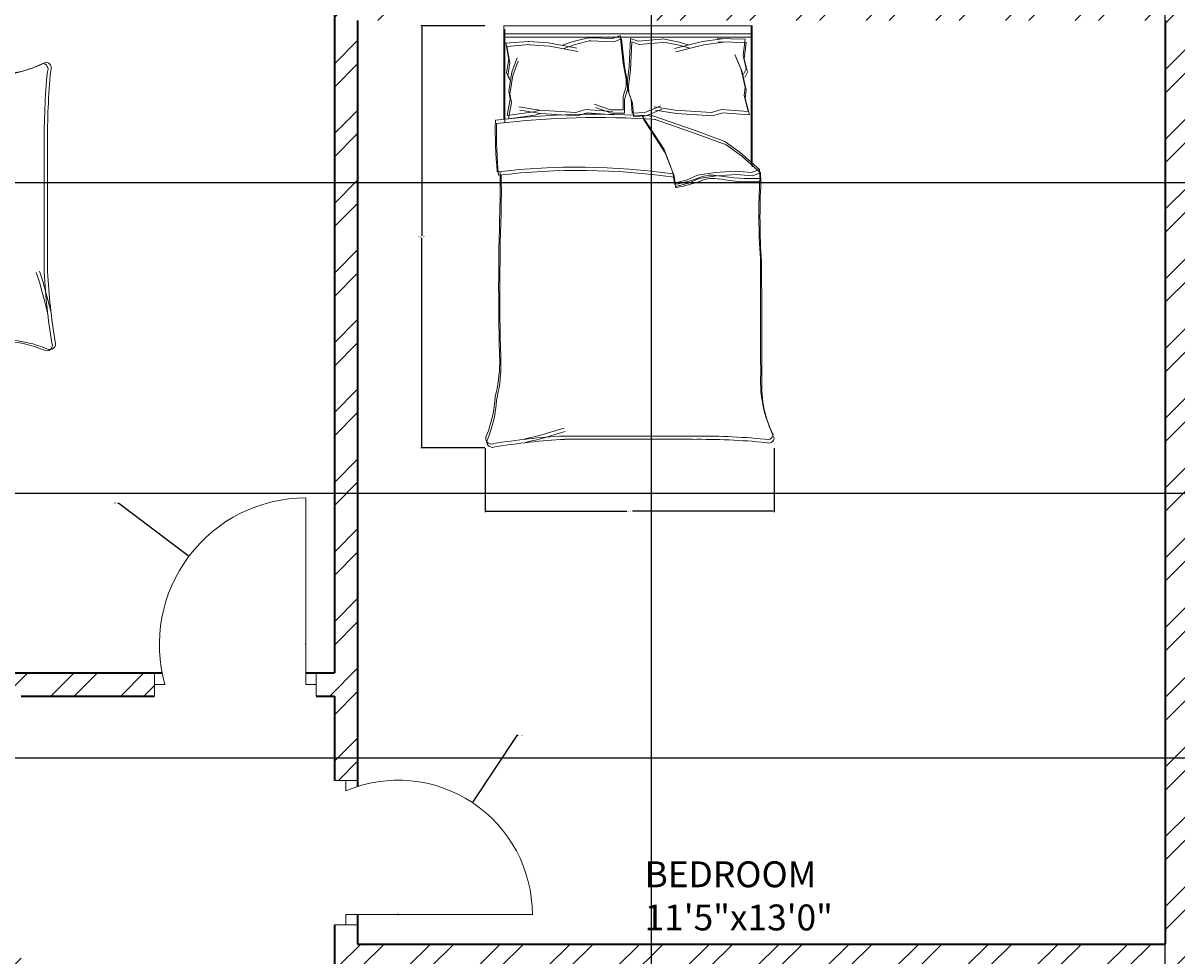
# Model space of a CAD drawing. Units: inches. Extents: x 2008 to 2657, y 1077 to 2165.
# Tile 12 of 16: x 2186 to 2409, y 1845 to 2025. Entities that reach past the tile are written whole.
import ezdxf

# ---------------------------------------------------------------- set-up
doc = ezdxf.new("R2010")
doc.units = ezdxf.units.IN
for name, color, linetype, lineweight in [('A-ANNO-DIMS', 2, 'Continuous', 18), ('A-AREA-IDEN', 4, 'Continuous', 18), ('A-DOOR', 11, 'Continuous', 18), ('A-FURN', 8, 'Continuous', 13), ('A-WALL', 7, 'Continuous', 35)]:
    doc.layers.add(name, color=color, linetype=linetype, lineweight=lineweight)
doc.layers.add('A-WALL-PATT', color=30, linetype='Continuous', lineweight=13, true_color=0xf8991e)
doc.styles.get("Standard").update_dxf_attribs({"font": 'arial.ttf'})
doc.dimstyles.get("Standard").update_dxf_attribs({"dimtxt": 0.18, "dimasz": 0.18, "dimexe": 0.18, "dimexo": 0.0625, "dimgap": 0.09, "dimtad": 0, "dimtih": 1, "dimtoh": 1, "dimdec": 4, "dimzin": 0, "dimdsep": 46, "dimtxsty": 'Standard', "dimcen": 0.09, "dimadec": 0, "dimazin": 0, "dimtfac": 1, "dimtdec": 4, "dimtofl": 0, "dimtmove": 0, "dimatfit": 3, "dimfxl": 1, "dimtolj": 1, "dimtzin": 0, "dimarcsym": 0})

# ---------------------------------------------------------------- blocks, each defined once
blk = doc.blocks.new('BED-DOUBLE')
for p, q in [((0, 51.49), (0.64, 51.49)), ((0, 3.48), (0, 51.49)), ((0, 51.27), (26.61, 51.27)), ((0, 51.27), (26.61, 51.27)), ((0.64, 51.49), (27.25, 51.49)), ((0.64, 51.49), (27.25, 51.49)), ((1.53, 3.48), (1.53, 51.27)), ((1.53, 3.48), (1.53, 51.27)), ((2.17, 3.7), (2.17, 51.49)), ((2.17, 3.7), (2.17, 51.49)), ((27.75, 52.87), (24.5, 49.16)), ((27.75, 52.87), (24.5, 49.16)), ((28.39, 53.1), (25.14, 49.39)), ((28.39, 53.1), (25.14, 49.39)), ((29.49, 52.95), (27.75, 52.87, 3.87)), ((29.49, 52.95), (27.75, 52.87, 3.87)), ((28.37, 51.33), (27.75, 52.87)), ((28.37, 51.33), (27.75, 52.87)), ((28.06, 48.23), (28.37, 51.33)), ((28.06, 48.23), (28.37, 51.33)), ((30.13, 53.18), (28.39, 53.1, 3.87)), ((30.13, 53.18), (28.39, 53.1, 3.87)), ((29, 51.56), (28.39, 53.1)), ((29, 51.56), (28.39, 53.1)), ((28.7, 48.46), (29, 51.56)), ((28.7, 48.46), (29, 51.56)), ((2.56, 50.11), (2.46, 44.71)), ((2.56, 50.11), (2.46, 44.71)), ((2.56, 50.11), (5.77, 49.73)), ((2.56, 50.11), (5.77, 49.73)), ((3.2, 50.34), (3.1, 44.94)), ((3.2, 50.34), (3.1, 44.94)), ((3.2, 50.34), (6.41, 49.96)), ((3.2, 50.34), (6.41, 49.96)), ((8.26, 49.31), (5.58, 48.13)), ((8.26, 49.31), (5.58, 48.13)), ((5.77, 49.73), (8.34, 50.33)), ((5.77, 49.73), (8.34, 50.33)), ((8.9, 49.54), (6.22, 48.36)), ((8.9, 49.54), (6.22, 48.36)), ((6.41, 49.96), (8.98, 50.56)), ((6.41, 49.96), (8.98, 50.56)), ((11.83, 50.11), (8.26, 49.31)), ((11.83, 50.11), (8.26, 49.31)), ((8.34, 50.33), (9.38, 49.82)), ((8.34, 50.33), (9.38, 49.81)), ((12.47, 50.34), (8.9, 49.54)), ((12.47, 50.34), (8.9, 49.54)), ((8.98, 50.56), (10.02, 50.04)), ((8.98, 50.56), (10.02, 50.04)), ((13.43, 49.92), (11.83, 50.11)), ((13.43, 49.92), (11.83, 50.11)), ((14.07, 50.15), (12.47, 50.34)), ((14.07, 50.15), (12.47, 50.34)), ((16.57, 50.7), (13.43, 49.92)), ((16.57, 50.7), (13.43, 49.92)), ((17.21, 50.93), (14.07, 50.15)), ((17.21, 50.93), (14.07, 50.15)), ((16.17, 45.57), (16.57, 50.7)), ((16.17, 45.57), (16.57, 50.7)), ((16.81, 45.8), (17.21, 50.93)), ((16.81, 45.8), (17.21, 50.93)), ((24.5, 49.16), (22.33, 46.22)), ((24.5, 49.16), (22.33, 46.22)), ((25.14, 49.39), (22.97, 46.45)), ((25.14, 49.39), (22.97, 46.45)), ((28.37, 44.36), (28.06, 48.23)), ((28.37, 44.36), (28.06, 48.23)), ((29, 44.59), (28.7, 48.46)), ((29, 44.59), (28.7, 48.46)), ((2.46, 44.71), (2.54, 45.71)), ((2.46, 44.71), (2.54, 45.71)), ((2.54, 45.71), (3.07, 41.91)), ((2.54, 45.71), (3.07, 41.91)), ((3.1, 44.94), (3.18, 45.94)), ((3.1, 44.94), (3.18, 45.94)), ((3.18, 45.94), (3.71, 42.14)), ((3.18, 45.94), (3.71, 42.14)), ((16.73, 43.61), (16.17, 45.57)), ((16.73, 43.61), (16.17, 45.57)), ((17.37, 43.84), (16.81, 45.8)), ((17.37, 43.83), (16.81, 45.8)), ((22.33, 46.22), (20.32, 40.64)), ((22.33, 46.22), (20.32, 40.64)), ((22.97, 46.45), (20.96, 40.87)), ((22.97, 46.45), (20.96, 40.87)), ((29.47, 41.18), (29, 44.59)), ((29.47, 41.18), (29, 44.59)), ((16.3, 36.6), (16.73, 43.61)), ((16.3, 36.6), (16.73, 43.61)), ((16.93, 36.83), (17.37, 43.84)), ((16.93, 36.82), (17.37, 43.83)), ((28.83, 40.95), (28.37, 44.36)), ((28.83, 40.95), (28.37, 44.36)), ((3.07, 41.91), (4.42, 36.5)), ((3.07, 41.91), (4.42, 36.5)), ((3.71, 42.14), (5.06, 36.72)), ((3.71, 42.14), (5.06, 36.72)), ((20.32, 40.64), (17.38, 32.31)), ((20.32, 40.64), (17.38, 32.31)), ((20.96, 40.87), (18.02, 32.54)), ((20.96, 40.87), (18.02, 32.53)), ((29.76, 38.94), (28.83, 40.95)), ((29.76, 38.94), (28.83, 40.95)), ((30.4, 39.17), (29.47, 41.18)), ((30.4, 39.17), (29.47, 41.18)), ((3.67, 39.2), (3.08, 37.14)), ((3.67, 39.2), (3.08, 37.14)), ((4.31, 39.43), (3.72, 37.36)), ((4.31, 39.43), (3.72, 37.36)), ((30.38, 36.46), (29.76, 38.94)), ((30.38, 36.46), (29.76, 38.94)), ((31.02, 36.69), (30.4, 39.17)), ((31.02, 36.69), (30.4, 39.17)), ((79.25, 15.06), (79.25, 39.68)), ((79.25, 15.06), (79.25, 39.68)), ((79.88, 15.29), (79.88, 39.91)), ((79.88, 15.29), (79.88, 39.91)), ((3.08, 37.14), (2.54, 34.21)), ((3.08, 37.14), (2.54, 34.2)), ((3.72, 37.36), (3.18, 34.43)), ((3.72, 37.36), (3.18, 34.43)), ((15.63, 32.56), (16.3, 36.6)), ((15.63, 32.56), (16.3, 36.6)), ((16.27, 32.79), (16.93, 36.83)), ((16.27, 32.79), (16.93, 36.82)), ((23.88, 34.45), (28.37, 36.15)), ((23.88, 34.45), (28.37, 36.15)), ((24.52, 34.68), (29, 36.38)), ((24.52, 34.68), (29, 36.38)), ((28.37, 36.15), (30.38, 36.46)), ((28.37, 36.15), (30.38, 36.46)), ((29, 36.38), (31.02, 36.69)), ((29, 36.38), (31.02, 36.69)), ((2.54, 34.21), (2.56, 33.88)), ((2.54, 34.2), (2.56, 33.88)), ((2.56, 33.88), (2.98, 29.46)), ((2.56, 33.88), (2.98, 29.46)), ((3.18, 34.43), (3.2, 34.11)), ((3.18, 34.43), (3.2, 34.11)), ((3.2, 34.11), (3.62, 29.68)), ((3.2, 34.11), (3.62, 29.68)), ((16.74, 30.75), (15.45, 33.82)), ((16.74, 30.75), (15.45, 33.82)), ((17.38, 30.98), (16.09, 34.05)), ((17.38, 30.98), (16.09, 34.05)), ((17.38, 30.26), (23.88, 34.45)), ((17.38, 30.26), (23.88, 34.45)), ((18.02, 30.49), (24.52, 34.68)), ((18.02, 30.49), (24.52, 34.68)), ((2.98, 29.46), (2.49, 27.98)), ((2.98, 29.46), (2.49, 27.98)), ((3.62, 29.68), (3.13, 28.21)), ((3.62, 29.68), (3.13, 28.21)), ((16.89, 28.3), (16.74, 30.75)), ((16.89, 28.3), (16.74, 30.75)), ((17.53, 28.53), (17.38, 30.98)), ((17.53, 28.53), (17.38, 30.98)), ((2.49, 27.98), (7.87, 27.73)), ((2.49, 27.98), (7.87, 27.73)), ((2.51, 26.21), (7.86, 26.79)), ((2.51, 26.21), (7.86, 26.79)), ((3.13, 28.21), (8.51, 27.96)), ((3.13, 28.21), (8.51, 27.96)), ((7.22, 26.56), (10.4, 27.14)), ((7.22, 26.56), (10.4, 27.14)), ((7.86, 26.79), (11.04, 27.37)), ((7.86, 26.79), (11.04, 27.37)), ((7.87, 27.73), (11.08, 27.36)), ((7.87, 27.73), (11.08, 27.36)), ((8.51, 27.96), (11.72, 27.58)), ((8.51, 27.96), (11.72, 27.58)), ((10.4, 27.14), (11.7, 27.14)), ((10.4, 27.14), (11.7, 27.14)), ((11.04, 27.37), (12.34, 27.37)), ((11.04, 27.37), (12.34, 27.37)), ((11.08, 27.36), (12.38, 27.44)), ((11.08, 27.36), (12.38, 27.44)), ((11.7, 27.14), (13.58, 26.56)), ((11.7, 27.14), (13.58, 26.56)), ((11.72, 27.58), (13.02, 27.66)), ((11.72, 27.58), (13.02, 27.66)), ((12.34, 27.37), (14.22, 26.79)), ((12.34, 27.37), (14.22, 26.79)), ((12.38, 27.44), (14.22, 28.13)), ((12.38, 27.44), (14.22, 28.13)), ((13.02, 27.66), (14.86, 28.36)), ((13.02, 27.66), (14.86, 28.36)), ((14.22, 28.13), (16.89, 28.3)), ((14.22, 28.13), (16.89, 28.3)), ((14.22, 26.79), (16.9, 26.79)), ((14.22, 26.79), (16.9, 26.79)), ((14.86, 28.36), (17.53, 28.53)), ((14.86, 28.36), (17.53, 28.53)), ((16.9, 26.79), (16.9, 24.33)), ((16.9, 26.79), (16.9, 24.33)), ((1.87, 25.98), (7.22, 26.56)), ((1.87, 25.98), (7.22, 26.56)), ((2.45, 24.54), (1.87, 25.98)), ((2.45, 24.54), (1.87, 25.98)), ((2.3, 20.09), (2.45, 24.54)), ((2.3, 20.09), (2.45, 24.54)), ((3.09, 24.77), (2.51, 26.21)), ((3.09, 24.77), (2.51, 26.21)), ((2.94, 20.32), (3.09, 24.77)), ((2.94, 20.32), (3.09, 24.77)), ((13.58, 26.56), (16.26, 26.56)), ((13.58, 26.56), (16.26, 26.56)), ((16.17, 19.38), (16.57, 24.52)), ((16.17, 19.38), (16.57, 24.52)), ((16.26, 26.56), (16.26, 24.1)), ((16.26, 26.56), (16.26, 24.1)), ((16.81, 19.61), (17.21, 24.74)), ((16.81, 19.61), (17.21, 24.74)), ((16.26, 24.1), (15.17, 20.96)), ((16.26, 24.1), (15.17, 20.96)), ((16.9, 24.33), (15.81, 21.19)), ((16.9, 24.33), (15.81, 21.19)), ((2.3, 19.77), (2.3, 20.09)), ((2.3, 19.77), (2.3, 20.09)), ((2.94, 20), (2.94, 20.32)), ((2.94, 20), (2.94, 20.32)), ((3.03, 16.88), (2.3, 19.77)), ((3.03, 16.88), (2.3, 19.77)), ((3.67, 17.11), (2.94, 20)), ((3.67, 17.11), (2.94, 20)), ((3.96, 12.34), (4.97, 17.83)), ((3.96, 12.34), (4.97, 17.83)), ((16.73, 17.42), (16.17, 19.38)), ((16.73, 17.42), (16.17, 19.38)), ((17.37, 17.65), (16.81, 19.61)), ((17.37, 17.65), (16.81, 19.61)), ((3.75, 14.86), (3.03, 16.88)), ((3.75, 14.86), (3.03, 16.88)), ((3.32, 12.11), (4.33, 17.6)), ((3.32, 12.11), (4.33, 17.6)), ((4.39, 15.08), (3.67, 17.11)), ((4.39, 15.08), (3.67, 17.11)), ((16.3, 10.41), (16.73, 17.42)), ((16.3, 10.41), (16.73, 17.42)), ((16.93, 10.64), (17.37, 17.65)), ((16.93, 10.64), (17.37, 17.65)), ((3.03, 8.29), (3.32, 12.11)), ((3.03, 8.29), (3.32, 12.11)), ((3.67, 8.51), (3.96, 12.34)), ((3.67, 8.51), (3.96, 12.34)), ((15.63, 6.38), (16.3, 10.41)), ((15.63, 6.38), (16.3, 10.41)), ((16.27, 6.61), (16.93, 10.64)), ((16.27, 6.61), (16.93, 10.64)), ((16.3, 10.41), (16.62, 9.28)), ((16.3, 10.41), (16.62, 9.28)), ((16.62, 9.28), (17.34, 4.18)), ((16.62, 9.28), (17.34, 4.18)), ((16.93, 10.64), (17.26, 9.51)), ((16.93, 10.64), (17.26, 9.51)), ((17.26, 9.51), (17.98, 4.41)), ((17.26, 9.51), (17.98, 4.41)), ((3.01, 8.18), (3.03, 8.29)), ((3.01, 8.18), (3.03, 8.29)), ((3.34, 3.9), (3.01, 8.18)), ((3.34, 3.9), (3.01, 8.18)), ((3.65, 8.41), (3.67, 8.51)), ((3.65, 8.41), (3.67, 8.51)), ((3.98, 4.13), (3.65, 8.41)), ((3.98, 4.13), (3.65, 8.41)), ((3.32, 3.9), (6.5, 4.47)), ((3.32, 3.89), (6.5, 4.47)), ((3.96, 4.12), (7.14, 4.7)), ((3.96, 4.12), (7.14, 4.7)), ((8.96, 5.05), (6.21, 6.06)), ((8.96, 5.05), (6.21, 6.06)), ((6.5, 4.47), (9.1, 4.04)), ((6.5, 4.47), (9.1, 4.04)), ((9.59, 5.28), (6.85, 6.29)), ((9.59, 5.28), (6.85, 6.29)), ((7.14, 4.7), (9.74, 4.27)), ((7.14, 4.7), (9.74, 4.27)), ((12.57, 4.47), (8.96, 5.05)), ((12.57, 4.47), (8.96, 5.05)), ((9.1, 4.04), (10.11, 4.62)), ((9.1, 4.04), (10.11, 4.62)), ((13.21, 4.7), (9.59, 5.28)), ((13.21, 4.7), (9.59, 5.28)), ((9.74, 4.27), (10.75, 4.85)), ((9.74, 4.27), (10.75, 4.85)), ((14.16, 4.76), (12.57, 4.47)), ((14.16, 4.76), (12.57, 4.47)), ((14.8, 4.99), (13.21, 4.7)), ((14.8, 4.99), (13.21, 4.7)), ((17.34, 4.18), (14.16, 4.76)), ((17.34, 4.18), (14.16, 4.76)), ((17.98, 4.41), (14.8, 4.99)), ((17.98, 4.41), (14.8, 4.99)), ((18.11, 3.48), (0, 3.48)), ((18.11, 3.48), (0, 3.48)), ((18.75, 3.7), (0.64, 3.7)), ((18.75, 3.7), (0.64, 3.7))]:
    blk.add_line(p, q)
for centre, radius, start, end in [((69.31, 76.39), 23.07, 267.4714, 296.4681), ((69.31, 76.39), 23.07, 267.4714, 296.4681), ((79.51, 54.64), 1.1, 332.6588, 86.02), ((79.51, 54.64), 1.1, 332.6588, 86.02), ((68.67, 76.16), 23.07, 267.4714, 296.4681), ((68.67, 76.16), 23.07, 267.4714, 296.4681), ((78.87, 54.41), 1.1, 332.6588, 86.02), ((78.87, 54.41), 1.1, 332.6588, 86.02), ((212.28, 41.15), 133.04, 174.4998, 180.6351), ((212.28, 41.15), 133.04, 174.4998, 180.6351), ((212.92, 41.38), 133.04, 174.4998, 180.6351), ((212.92, 41.38), 133.04, 174.4998, 180.6351), ((-6.66, 51.33), 36.18, 349.8763, 2.5657), ((-6.66, 51.33), 36.18, 349.8763, 2.5657), ((36.32, 182.27), 129.5, 266.9791, 273.8365), ((36.32, 182.27), 129.5, 266.9791, 273.8365), ((-6.02, 51.56), 36.18, 349.8763, 2.5657), ((-6.02, 51.56), 36.18, 349.8763, 2.5657), ((36.95, 182.49), 129.5, 266.9791, 273.8365), ((36.95, 182.49), 129.5, 266.9791, 273.8365), ((67.82, -4508.74), 4561.86, 90.00217, 90.28689), ((67.82, -4508.74), 4561.86, 90.00217, 90.28689), ((68.46, -4508.51), 4561.86, 90.00217, 90.28689), ((68.46, -4508.51), 4561.86, 90.00217, 90.28689), ((35.07, 43.74), 6.22, 168.6608, 203.7384), ((35.07, 43.74), 6.22, 168.6608, 203.7384), ((35.71, 43.97), 6.22, 168.6608, 203.7384), ((35.71, 43.97), 6.22, 168.6608, 203.7384), ((1.48, 31.15), 29.65, 10.6617, 19.8806), ((1.48, 31.15), 29.65, 10.6617, 19.8806), ((2.12, 31.38), 29.65, 10.6617, 19.8806), ((2.12, 31.38), 29.65, 10.6617, 19.8806), ((156.32, 17.76), 129.02, 171.7845, 186.9006), ((156.32, 17.76), 129.02, 171.7845, 186.9006), ((156.96, 17.98), 129.02, 171.7845, 186.9006), ((156.96, 17.98), 129.02, 171.7845, 186.9006), ((30.44, 36.64), 0.185, 250.2464, 1.1377), ((30.44, 36.64), 0.185, 250.2464, 1.1377), ((31.08, 36.87), 0.185, 250.2464, 1.1377), ((31.08, 36.86), 0.185, 250.2464, 1.1377), ((182.05, 21.36), 164.97, 176.0865, 186.7821), ((182.05, 21.36), 164.97, 176.0865, 186.7821), ((182.69, 21.59), 164.97, 176.0865, 186.7821), ((182.69, 21.59), 164.97, 176.0865, 186.7821), ((-23.71, -17.22), 106.46, 13.3832, 17.7053), ((-23.71, -17.22), 106.46, 13.3832, 17.7053), ((-23.07, -16.99), 106.46, 13.3832, 17.7053), ((-23.07, -16.99), 106.46, 13.3832, 17.7053), ((200.84, 21.43), 121.76, 182.9958, 189.4091), ((200.84, 21.43), 121.76, 182.9958, 189.4091), ((201.48, 21.66), 121.76, 182.9958, 189.4091), ((201.48, 21.66), 121.76, 182.9958, 189.4091), ((20.1, 85.16), 83.31, 268.7218, 275.604), ((20.1, 85.16), 83.31, 268.7218, 275.604), ((20.74, 85.39), 83.31, 268.7218, 275.604), ((20.74, 85.39), 83.31, 268.7218, 275.604), ((31.17, -167.31), 170.11, 88.4762, 91.0082), ((31.17, -167.31), 170.11, 88.4762, 91.0082), ((31.81, -167.08), 170.11, 88.4762, 91.0082), ((31.81, -167.08), 170.11, 88.4762, 91.0082), ((50.61, 484.82), 482.31, 268.2277, 271.7185), ((50.61, 484.82), 482.31, 268.2277, 271.7185), ((51.25, 485.05), 482.31, 268.2277, 271.7185), ((51.25, 485.05), 482.31, 268.2277, 271.7185), ((64.52, -26.9), 29.63, 76.0648, 88.9113), ((64.52, -26.9), 29.63, 76.0648, 88.9113), ((65.15, -26.67), 29.63, 76.0648, 88.9113), ((65.15, -26.67), 29.63, 76.0648, 88.9113), ((70.28, -21.66), 23.56, 67.9751, 86.652), ((70.28, -21.66), 23.56, 67.9751, 86.652), ((70.92, -21.43), 23.56, 67.9751, 86.652), ((70.92, -21.43), 23.56, 67.9751, 86.652), ((79.72, 1.09), 1.09, 236.1736, 23.4781), ((79.72, 1.09), 1.09, 236.1736, 23.4781), ((80.36, 1.32), 1.09, 236.1736, 23.4781), ((80.36, 1.32), 1.09, 236.1736, 23.4781)]:
    blk.add_arc(centre, radius, start, end)
blk = doc.blocks.new('*D11')
at = {"layer": 'A-ANNO-DIMS', "color": 0, "lineweight": -2, "transparency": 16777216}
for p, q in [((2275.34, 2024.63), (2262.99, 2024.63)), ((2263.17, 2024.45), (2263.17, 1984.04)), ((2263.17, 1943.27), (2263.17, 1983.68)), ((2275.34, 1943.09), (2262.99, 1943.09))]:
    blk.add_line(p, q, dxfattribs=at)
at = {"layer": 'A-ANNO-DIMS', "color": 0, "transparency": 16777216}
for points in [[(2263.14, 2024.45), (2263.2, 2024.45), (2263.17, 2024.63)], [(2263.14, 1943.27), (2263.2, 1943.27), (2263.17, 1943.09)]]:
    blk.add_solid(points, dxfattribs=at)
at = {"layer": 'Defpoints', "color": 0, "transparency": 16777216}
for p in [(2275.4, 2024.63), (2263.17, 1943.09), (2275.4, 1943.09)]:
    blk.add_point(p, dxfattribs=at)
at = {"layer": 'A-ANNO-DIMS', "color": 0, "transparency": 16777216, "insert": (2263.17, 1983.86), "char_height": 0.18, "attachment_point": 5}
blk.add_mtext('\\A1;BED 82 TYP.', dxfattribs=at)
blk = doc.blocks.new('*D12')
at = {"layer": 'A-ANNO-DIMS', "color": 0, "lineweight": -2, "transparency": 16777216}
for p, q in [((2275.4, 1943.02), (2275.4, 1930.67)), ((2331.23, 1943.02), (2331.23, 1930.67)), ((2275.58, 1930.85), (2302.79, 1930.85)), ((2331.05, 1930.85), (2303.84, 1930.85))]:
    blk.add_line(p, q, dxfattribs=at)
at = {"layer": 'A-ANNO-DIMS', "color": 0, "transparency": 16777216}
for points in [[(2275.58, 1930.88), (2275.58, 1930.82), (2275.4, 1930.85)], [(2331.05, 1930.88), (2331.05, 1930.82), (2331.23, 1930.85)]]:
    blk.add_solid(points, dxfattribs=at)
at = {"layer": 'Defpoints', "color": 0, "transparency": 16777216}
for p in [(2275.4, 1943.09), (2331.23, 1943.09), (2331.23, 1930.85)]:
    blk.add_point(p, dxfattribs=at)
at = {"layer": 'A-ANNO-DIMS', "color": 0, "transparency": 16777216, "insert": (2303.32, 1930.85), "char_height": 0.18, "attachment_point": 5}
blk.add_mtext('\\A1;56 TYP.', dxfattribs=at)
blk = doc.blocks.new('*D51')
at = {"layer": 'A-ANNO-DIMS', "color": 0, "lineweight": -2, "transparency": 16777216}
for p, q in [((2307.5, 1617.74), (2307.5, 2142.9)), ((2307.68, 2142.72), (2356.74, 2142.72)), ((2406.58, 2142.72), (2357.53, 2142.72)), ((2406.76, 1617.74), (2406.76, 2142.9))]:
    blk.add_line(p, q, dxfattribs=at)
at = {"layer": 'A-ANNO-DIMS', "color": 0, "transparency": 16777216}
for points in [[(2307.68, 2142.75), (2307.68, 2142.69), (2307.5, 2142.72)], [(2406.58, 2142.75), (2406.58, 2142.69), (2406.76, 2142.72)]]:
    blk.add_solid(points, dxfattribs=at)
at = {"layer": 'Defpoints', "color": 0, "transparency": 16777216}
for p in [(2406.76, 2142.72), (2307.5, 1617.67), (2406.76, 1617.67)]:
    blk.add_point(p, dxfattribs=at)
at = {"layer": 'A-ANNO-DIMS', "color": 0, "transparency": 16777216, "insert": (2357.13, 2142.72), "char_height": 0.18, "attachment_point": 5}
blk.add_mtext('\\A1;99.26', dxfattribs=at)
blk = doc.blocks.new('*D66')
at = {"layer": 'A-ANNO-DIMS', "color": 0, "lineweight": -2, "transparency": 16777216}
for p, q in [((2572.2, 2055.67), (2028.03, 2055.67)), ((2028.21, 2055.49), (2028.21, 2025.16)), ((2028.21, 1994.47), (2028.21, 2024.8)), ((2572.2, 1994.29), (2028.03, 1994.29))]:
    blk.add_line(p, q, dxfattribs=at)
at = {"layer": 'A-ANNO-DIMS', "color": 0, "transparency": 16777216}
for points in [[(2028.18, 2055.49), (2028.24, 2055.49), (2028.21, 2055.67)], [(2028.18, 1994.47), (2028.24, 1994.47), (2028.21, 1994.29)]]:
    blk.add_solid(points, dxfattribs=at)
at = {"layer": 'Defpoints', "color": 0, "transparency": 16777216}
for p in [(2572.26, 2055.67), (2028.21, 1994.29), (2572.26, 1994.29)]:
    blk.add_point(p, dxfattribs=at)
at = {"layer": 'A-ANNO-DIMS', "color": 0, "transparency": 16777216, "insert": (2028.21, 2024.98), "char_height": 0.18, "attachment_point": 5}
blk.add_mtext('\\A1;61.39', dxfattribs=at)
blk = doc.blocks.new('*D67')
at = {"layer": 'A-ANNO-DIMS', "color": 0, "lineweight": -2, "transparency": 16777216}
for p, q in [((2572.2, 1934.29), (2028.03, 1934.29)), ((2028.21, 1934.11), (2028.21, 1908.91)), ((2028.21, 1883.35), (2028.21, 1908.55)), ((2572.2, 1883.17), (2028.03, 1883.17))]:
    blk.add_line(p, q, dxfattribs=at)
at = {"layer": 'A-ANNO-DIMS', "color": 0, "transparency": 16777216}
for points in [[(2028.18, 1934.11), (2028.24, 1934.11), (2028.21, 1934.29)], [(2028.18, 1883.35), (2028.24, 1883.35), (2028.21, 1883.17)]]:
    blk.add_solid(points, dxfattribs=at)
at = {"layer": 'Defpoints', "color": 0, "transparency": 16777216}
for p in [(2028.21, 1934.29), (2572.26, 1934.29), (2572.26, 1883.17)]:
    blk.add_point(p, dxfattribs=at)
at = {"layer": 'A-ANNO-DIMS', "color": 0, "transparency": 16777216, "insert": (2028.21, 1908.73), "char_height": 0.18, "attachment_point": 5}
blk.add_mtext('\\A1;51.11', dxfattribs=at)
blk = doc.blocks.new('*D74')
at = {"layer": 'A-ANNO-DIMS', "color": 0, "lineweight": -2, "transparency": 16777216}
for p, q in [((2204.47, 1932.42), (2204.65, 1932.42)), ((2204.65, 1932.42), (2218.04, 1922.3)), ((2240.66, 1905.15), (2240.84, 1905.15)), ((2240.75, 1905.06), (2240.75, 1905.24))]:
    blk.add_line(p, q, dxfattribs=at)
at = {"layer": 'A-ANNO-DIMS', "color": 0, "transparency": 16777216}
blk.add_solid([(2218.06, 1922.33), (2218.02, 1922.28), (2218.18, 1922.19)], dxfattribs=at)
at = {"layer": 'Defpoints', "color": 0, "transparency": 16777216}
for p in [(2218.18, 1922.19), (2240.75, 1905.15)]:
    blk.add_point(p, dxfattribs=at)
at = {"layer": 'A-ANNO-DIMS', "color": 0, "transparency": 16777216, "insert": (2203.99, 1932.42), "char_height": 0.18, "attachment_point": 5}
blk.add_mtext('\\A1;R28.28', dxfattribs=at)
blk = doc.blocks.new('*D79')
at = {"layer": 'A-ANNO-DIMS', "color": 0, "lineweight": -2, "transparency": 16777216}
for p, q in [((2281.52, 1887.55), (2273.02, 1874.74)), ((2281.7, 1887.55), (2281.52, 1887.55)), ((2258.5, 1852.99), (2258.68, 1852.99)), ((2258.59, 1852.9), (2258.59, 1853.08))]:
    blk.add_line(p, q, dxfattribs=at)
at = {"layer": 'A-ANNO-DIMS', "color": 0, "transparency": 16777216}
blk.add_solid([(2272.99, 1874.76), (2273.04, 1874.72), (2272.92, 1874.59)], dxfattribs=at)
at = {"layer": 'Defpoints', "color": 0, "transparency": 16777216}
for p in [(2272.92, 1874.59), (2258.59, 1852.99)]:
    blk.add_point(p, dxfattribs=at)
at = {"layer": 'A-ANNO-DIMS', "color": 0, "transparency": 16777216, "insert": (2282.25, 1887.55), "char_height": 0.18, "attachment_point": 5}
blk.add_mtext('\\A1;R25.923', dxfattribs=at)

msp = doc.modelspace()

# ---------------------------------------------------------------- hatches: boundary and pattern name
at = {"layer": 'A-WALL-PATT'}
h = msp.add_hatch(dxfattribs=at)
h.set_pattern_fill('ANSI32', color=256)
h.paths.add_polyline_path([(2109.2619, 2094.6743), (2104.7619, 2094.6743), (2104.7619, 2072.1743), (2104.7619, 2021.6151), (2109.2619, 2021.6151), (2109.2619, 2055.6743), (2126.1387, 2055.6743), (2126.1387, 2057.9243), (2126.1387, 2060.1743), (2109.2619, 2060.1743)])
h.paths.add_polyline_path([(2223.2494, 2057.9243), (2223.2494, 2060.1743), (2186.1387, 2060.1743), (2186.1387, 2055.6743), (2223.2494, 2055.6743)])
h.paths.add_polyline_path([(2250.7619, 2072.1743), (2250.7619, 2090.1743), (2250.7619, 2094.6743), (2246.2619, 2094.6743), (2246.2619, 2060.1743), (2242.7242, 2060.1743), (2242.7242, 2055.6743), (2246.2619, 2055.6743), (2246.2619, 1899.6743), (2242.7458, 1899.6743), (2242.7458, 1897.4243), (2242.7458, 1895.1743), (2246.2619, 1895.1743), (2246.2619, 1878.8745), (2248.5119, 1878.8745), (2250.7619, 1878.8745), (2250.7619, 1991.1743), (2250.7619, 2025.6743), (2257.6798, 2025.6743), (2257.6798, 2027.9243), (2257.6798, 2030.1743), (2250.7619, 2030.1743)])
h.paths.add_polyline_path([(2411.2619, 2031.6743), (2409.0119, 2031.6743), (2406.7619, 2031.6743), (2406.7619, 2030.1743), (2322.7619, 2030.1743), (2322.7619, 2053.3443), (2318.2619, 2053.3443), (2318.2619, 2030.1743), (2305.6798, 2030.1743), (2305.6798, 2025.6743), (2318.2619, 2025.6743), (2322.7619, 2025.6743), (2406.7619, 2025.6743), (2406.7619, 1995.6743), (2406.7619, 1847.2677), (2250.7619, 1847.2677), (2250.7619, 1850.9902), (2248.5119, 1850.9902), (2246.2619, 1850.9902), (2246.2619, 1847.1743), (2246.2619, 1842.7677), (2303.0015, 1842.7677), (2303.0015, 1667.2413), (2298.4208, 1667.2413), (2298.4208, 1662.7413), (2303.0015, 1662.7413), (2303.0015, 1649.8758), (2307.5015, 1649.8758), (2307.5015, 1842.7677), (2406.7619, 1842.7677), (2411.2619, 1842.7677), (2411.2619, 1878.6743), (2415.8196, 1878.6743), (2415.8196, 1880.9243), (2415.8196, 1883.1743), (2411.2619, 1883.1743)])
h.paths.add_polyline_path([(2411.2619, 2094.6743), (2406.7619, 2094.6743), (2318.2619, 2094.6743), (2318.2619, 2077.3443), (2322.7619, 2077.3443), (2322.7619, 2090.1743), (2406.7619, 2090.1743), (2406.7619, 2072.1743), (2406.7619, 2067.6743), (2406.7619, 2052.7524), (2411.2619, 2052.7524), (2411.2619, 2055.6743), (2414.9888, 2055.6743), (2414.9888, 2057.9243), (2414.9888, 2060.1743), (2411.2619, 2060.1743), (2411.2619, 2072.1743)])
h.paths.add_polyline_path([(2576.7619, 2072.1743), (2576.7619, 2094.6743), (2572.2619, 2094.6743), (2572.2619, 2060.1743), (2525.8113, 2060.1743), (2525.8113, 2055.6743), (2572.2619, 2055.6743), (2572.2619, 1994.289), (2576.7619, 1994.289)])
h.paths.add_polyline_path([(2465.8113, 2060.1743), (2436.2802, 2060.1743), (2436.2802, 2055.6743), (2465.8113, 2055.6743), (2465.8113, 2057.9243)])
h.paths.add_polyline_path([(2576.7619, 1934.289), (2574.5119, 1934.289), (2572.2619, 1934.289), (2572.2619, 1883.1743), (2447.7027, 1883.1743), (2447.7027, 1878.6743), (2459.7619, 1878.6743), (2459.7619, 1830.4982), (2464.2619, 1830.4982), (2464.2619, 1878.6743), (2572.2619, 1878.6743), (2572.2619, 1868.4883), (2576.7619, 1868.4883)])
h.paths.add_polyline_path([(2576.7619, 1832.4883), (2572.2619, 1832.4883), (2572.2619, 1806.6743), (2464.2619, 1806.6743), (2464.2619, 1809.6629), (2459.7619, 1809.6629), (2459.7619, 1802.1743), (2483.7619, 1802.1743), (2483.7619, 1778.1743), (2488.2619, 1778.1743), (2488.2619, 1802.1743), (2572.2619, 1802.1743), (2572.2619, 1793.6101), (2576.7619, 1793.6101)])
h.paths.add_polyline_path([(2576.7619, 1769.6101), (2572.2619, 1769.6101), (2572.2619, 1754.1743), (2488.2619, 1754.1743), (2488.2619, 1757.2675), (2486.0119, 1757.2675), (2483.7619, 1757.2675), (2483.7619, 1754.1743), (2447.4528, 1754.1743), (2447.4528, 1749.6743), (2483.7619, 1749.6743), (2572.2619, 1749.6743), (2572.2619, 1715.1837), (2576.7619, 1715.1837)])
h.paths.add_polyline_path([(2576.7619, 1655.1837), (2572.2619, 1655.1837), (2572.2619, 1617.6743), (2411.2619, 1617.6743), (2411.2619, 1749.6743), (2414.2827, 1749.6743), (2414.2827, 1754.1743), (2406.7619, 1754.1743), (2406.7619, 1749.6743), (2406.7619, 1617.6743), (2307.5015, 1617.6743), (2307.5015, 1621.0007), (2305.2515, 1621.0007), (2303.0015, 1621.0007), (2303.0015, 1609.6944), (2307.5015, 1609.6944), (2307.5015, 1613.1743), (2406.7619, 1613.1743), (2406.7619, 1476.6743), (2415.532, 1476.6743), (2415.532, 1478.9243), (2415.532, 1481.1743), (2411.2619, 1481.1743), (2411.2619, 1613.1743), (2572.2619, 1613.1743), (2572.2619, 1584.6086), (2576.7619, 1584.6086)])
h.paths.add_polyline_path([(2576.7619, 1524.6086), (2572.2619, 1524.6086), (2572.2619, 1481.1743), (2483.7619, 1481.1743), (2447.5119, 1481.1743), (2447.5119, 1476.6743), (2483.7619, 1476.6743), (2483.7619, 1473.5051), (2488.2619, 1473.5051), (2488.2619, 1476.6743), (2572.2619, 1476.6743), (2572.2619, 1469.5488), (2576.7619, 1469.5488)])
h.paths.add_polyline_path([(2576.7619, 1445.5488), (2572.2619, 1445.5488), (2572.2619, 1428.6743), (2488.2619, 1428.6743), (2488.2619, 1455.6743), (2486.0119, 1455.6743), (2483.7619, 1455.6743), (2483.7619, 1428.6743), (2459.7619, 1428.6743), (2459.7619, 1422.1519), (2464.2619, 1422.1519), (2464.2619, 1424.1743), (2572.2619, 1424.1743), (2572.2619, 1407.5685), (2576.7619, 1407.5685)])
h.paths.add_polyline_path([(2576.7619, 1371.5685), (2572.2619, 1371.5685), (2572.2619, 1352.1743), (2464.2619, 1352.1743), (2464.2619, 1403.1384), (2462.0119, 1403.1384), (2459.7619, 1403.1384), (2459.7619, 1352.1743), (2446.3194, 1352.1743), (2446.3194, 1347.6743), (2572.2619, 1347.6743), (2572.2619, 1321.0291), (2576.7619, 1321.0291)])
h.paths.add_polyline_path([(2462.703, 1227.6743), (2436.0298, 1227.6743), (2436.0298, 1225.4243), (2436.0298, 1223.1743), (2462.703, 1223.1743), (2462.703, 1225.4243)])
h.paths.add_polyline_path([(2576.7619, 1261.0291), (2574.5119, 1261.0291), (2572.2619, 1261.0291), (2572.2619, 1227.6743), (2522.703, 1227.6743), (2522.703, 1223.1743), (2572.2619, 1223.1743), (2572.2619, 1188.6743), (2576.7619, 1188.6743), (2576.7619, 1193.1743), (2576.7619, 1223.1743)])
h.paths.add_polyline_path([(2414.2823, 1227.6743), (2411.2619, 1227.6743), (2411.2619, 1267.1779), (2409.0119, 1267.1779), (2406.7619, 1267.1779), (2406.7619, 1227.6743), (2322.7619, 1227.6743), (2322.7619, 1244.3623), (2318.2619, 1244.3623), (2318.2619, 1223.1743), (2406.7619, 1223.1743), (2406.7619, 1193.1743), (2406.7619, 1188.6743), (2411.2619, 1188.6743), (2411.2619, 1193.1743), (2411.2619, 1223.1743), (2414.2823, 1223.1743)])
h.paths.add_polyline_path([(2411.2619, 1347.6743), (2414.702, 1347.6743), (2414.702, 1349.9243), (2414.702, 1352.1743), (2411.2619, 1352.1743), (2411.2619, 1416.7413), (2307.5015, 1416.7413), (2307.5015, 1579.8489), (2305.2515, 1579.8489), (2303.0015, 1579.8489), (2303.0015, 1566.7413), (2299.2719, 1566.7413), (2299.2719, 1562.2413), (2303.0015, 1562.2413), (2303.0015, 1416.7413), (2246.2619, 1416.7413), (2246.2619, 1409.8616), (2250.7619, 1409.8616), (2250.7619, 1412.2413), (2406.7619, 1412.2413), (2406.7619, 1292.1743), (2304.9703, 1292.1743), (2304.9703, 1287.6743), (2318.2619, 1287.6743), (2318.2619, 1268.3623), (2322.7619, 1268.3623), (2322.7619, 1287.6743), (2406.7619, 1287.6743), (2406.7619, 1285.4748), (2411.2619, 1285.4748)])
h.paths.add_polyline_path([(2109.2619, 1262.7482), (2104.7619, 1262.7482), (2104.7619, 1223.1743), (2104.7619, 1193.1743), (2104.7619, 1188.6743), (2109.2619, 1188.6743), (2109.2619, 1223.1743), (2126.7928, 1223.1743), (2126.7928, 1225.4243), (2126.7928, 1227.6743), (2109.2619, 1227.6743)])
h.paths.add_polyline_path([(2222.3268, 1227.6743), (2186.7928, 1227.6743), (2186.7928, 1223.1743), (2222.3268, 1223.1743)])
h.paths.add_polyline_path([(2250.7619, 1287.6743), (2256.9703, 1287.6743), (2256.9703, 1289.9243), (2256.9703, 1292.1743), (2250.7619, 1292.1743), (2250.7619, 1382.2078), (2248.5119, 1382.2078), (2246.2619, 1382.2078), (2246.2619, 1347.6743), (2246.2619, 1227.6743), (2242.6068, 1227.6743), (2242.6068, 1223.1743), (2246.2619, 1223.1743), (2246.2619, 1188.6743), (2250.7619, 1188.6743), (2250.7619, 1193.1743), (2250.7619, 1227.6743)])
h.paths.add_polyline_path([(2133.2619, 1349.9243), (2133.2619, 1352.1743), (2109.2619, 1352.1743), (2109.2619, 1375.2826), (2104.7619, 1375.2826), (2104.7619, 1322.7482), (2109.2619, 1322.7482), (2109.2619, 1347.6743), (2133.2619, 1347.6743)])
h.paths.add_polyline_path([(2210.2105, 1352.1743), (2161.7619, 1352.1743), (2161.7619, 1412.2413), (2185.7619, 1412.2413), (2185.7619, 1420.1851), (2183.5119, 1420.1851), (2181.2619, 1420.1851), (2181.2619, 1416.7413), (2109.2619, 1416.7413), (2109.2619, 1452.4006), (2104.7619, 1452.4006), (2104.7619, 1399.2826), (2109.2619, 1399.2826), (2109.2619, 1412.2413), (2157.2619, 1412.2413), (2157.2619, 1352.1743), (2154.3383, 1352.1743), (2154.3383, 1347.6743), (2210.2105, 1347.6743)])
h.paths.add_polyline_path([(2185.7619, 1514.2413), (2161.7619, 1514.2413), (2161.7619, 1518.1307), (2159.5119, 1518.1307), (2157.2619, 1518.1307), (2157.2619, 1514.2413), (2109.2619, 1514.2413), (2109.2619, 1528.997), (2107.0119, 1528.997), (2104.7619, 1528.997), (2104.7619, 1488.4006), (2109.2619, 1488.4006), (2109.2619, 1509.7413), (2181.2619, 1509.7413), (2181.2619, 1441.2042), (2185.7619, 1441.2042)])
h.paths.add_polyline_path([(2270.4025, 1566.7413), (2109.2619, 1566.7413), (2080.7619, 1566.7413), (2080.7619, 1586.5643), (2076.2619, 1586.5643), (2076.2619, 1562.2413), (2080.7619, 1562.2413), (2104.7619, 1562.2413), (2104.7619, 1552.997), (2109.2619, 1552.997), (2109.2619, 1562.2413), (2157.2619, 1562.2413), (2157.2619, 1538.2413), (2161.7619, 1538.2413), (2161.7619, 1562.2413), (2205.2619, 1562.2413), (2270.4025, 1562.2413)])
h.paths.add_polyline_path([(2131.6813, 1897.4243), (2131.6813, 1899.6743), (2109.2619, 1899.6743), (2109.2619, 1961.6151), (2104.7619, 1961.6151), (2104.7619, 1886.8042), (2109.2619, 1886.8042), (2109.2619, 1895.1743), (2131.6813, 1895.1743)])
h.paths.add_polyline_path([(2185.7619, 1847.1743), (2161.7619, 1847.1743), (2161.7619, 1895.1743), (2185.7619, 1895.1743), (2211.543, 1895.1743), (2211.543, 1897.4243), (2211.543, 1899.6743), (2154.0916, 1899.6743), (2154.0916, 1897.4243), (2154.0916, 1895.1743), (2157.2619, 1895.1743), (2157.2619, 1847.1743), (2109.2619, 1847.1743), (2109.2619, 1862.8042), (2104.7619, 1862.8042), (2104.7619, 1821.243), (2109.2619, 1821.243), (2109.2619, 1842.6743), (2181.2619, 1842.6743), (2181.2619, 1840.6763), (2185.7619, 1840.6763)])
h.paths.add_polyline_path([(2109.2619, 1785.243), (2104.7619, 1785.243), (2104.7619, 1715.4691), (2109.2619, 1715.4691), (2109.2619, 1730.8423), (2157.2619, 1730.8423), (2157.2619, 1727.6404), (2161.7619, 1727.6404), (2161.7619, 1730.8423), (2185.7619, 1730.8423), (2185.7619, 1822.1438), (2183.5119, 1822.1438), (2181.2619, 1822.1438), (2181.2619, 1735.3423), (2109.2619, 1735.3423)])
h.paths.add_polyline_path([(2109.2619, 1691.4691), (2104.7619, 1691.4691), (2104.7619, 1667.2413), (2076.2619, 1667.2413), (2076.2619, 1646.5643), (2080.7619, 1646.5643), (2080.7619, 1662.7413), (2109.2619, 1662.7413), (2271.4941, 1662.7413), (2271.4941, 1664.9913), (2271.4941, 1667.2413), (2181.2619, 1667.2413), (2161.7619, 1667.2413), (2161.7619, 1708.3752), (2159.5119, 1708.3752), (2157.2619, 1708.3752), (2157.2619, 1667.2413), (2109.2619, 1667.2413)])
h.paths.add_polyline_path([(2233.1467, 1747.4973), (2270.0737, 1747.4973), (2270.0737, 1766.1547), (2233.1467, 1766.1547)], flags=9)

# ---------------------------------------------------------------- linework, layer by layer
at = {"layer": 'A-DOOR'}
for p, q in [((2240.7458, 1897.4243), (2240.7458, 1933.4243)), ((2211.543, 1899.6743), (2211.543, 1895.1743)), ((2242.7458, 1895.1743), (2242.7458, 1899.6743)), ((2242.7458, 1899.6743), (2242.7458, 1897.4243)), ((2211.543, 1895.1743), (2211.543, 1897.4243)), ((2211.543, 1897.4243), (2213.543, 1897.4243)), ((2242.7458, 1897.4243), (2240.7458, 1897.4243)), ((2250.7619, 1878.8745), (2246.2619, 1878.8745)), ((2246.2619, 1878.8745), (2248.5119, 1878.8745)), ((2248.5119, 1878.8745), (2248.5119, 1876.8745)), ((2248.5119, 1850.9902), (2248.5119, 1852.9902)), ((2248.5119, 1852.9902), (2284.5119, 1852.9902)), ((2246.2619, 1850.9902), (2250.7619, 1850.9902)), ((2250.7619, 1850.9902), (2248.5119, 1850.9902))]:
    msp.add_line(p, q, dxfattribs=at)
for centre, radius, start, end in [((2240.7458, 1905.1467), 28.2776, 90, 195.848313), ((2258.5888, 1852.9902), 25.9231, 0, 112.875203)]:
    msp.add_arc(centre, radius, start, end, dxfattribs=at)
at = {"layer": 'A-WALL'}
for p, q in [((2246.2619, 2055.6743), (2246.2619, 1899.6743)), ((2250.7619, 2025.6743), (2250.7619, 1877.7035)), ((2406.7619, 2025.6743), (2406.7619, 1995.6743)), ((2406.7619, 2003.1743), (2406.7619, 1847.2677)), ((2250.7619, 1991.1743), (2250.7619, 1877.7035)), ((2154.0916, 1899.6743), (2213.0027, 1899.6743)), ((2240.7458, 1899.6743), (2246.2619, 1899.6743)), ((2185.7619, 1895.1743), (2211.543, 1895.1743)), ((2242.7458, 1895.1743), (2246.2619, 1895.1743)), ((2246.2619, 1895.1743), (2246.2619, 1878.8745)), ((2250.7619, 1852.9902), (2250.7619, 1847.2677)), ((2246.2619, 1850.9902), (2246.2619, 1847.1743)), ((2246.2619, 1847.1743), (2246.2619, 1842.7677)), ((2250.7619, 1847.2677), (2406.7619, 1847.2677))]:
    msp.add_line(p, q, dxfattribs=at)

# ---------------------------------------------------------------- block references
at = {"layer": 'A-FURN', "rotation": 269.9999998331857}
msp.add_blockref('BED-DOUBLE', (2275.4901, 2024.6345), dxfattribs=at)
at = {"layer": 'A-FURN'}
msp.add_blockref('BED-DOUBLE', (2110.986, 1961.847), dxfattribs=at)

# ---------------------------------------------------------------- texts
at = {"layer": 'A-AREA-IDEN', "insert": (2306.1871, 1863.2351), "char_height": 5, "attachment_point": 1}
msp.add_mtext_dynamic_manual_height_columns('BEDROOM\\P11\'5"x13\'0"', width=161.06324, gutter_width=12.5, heights=[0], dxfattribs=at)

# ---------------------------------------------------------------- dimensions: what is measured, and where the dimension line sits
at = {"layer": 'A-ANNO-DIMS'}
dim = msp.add_linear_dim(base=(2406.7619, 2142.7243), p1=(2307.5015, 1617.6743), p2=(2406.7619, 1617.6743), dimstyle='Standard', override={"dimdec": 2, "dimlfac": 1, "dimrnd": 0, "dimzin": 0, "dimdsep": 46, "dimlunit": 2}, dxfattribs=at)
dim.commit()
dim.dimension.update_dxf_attribs({"geometry": '*D51', "text_midpoint": (2357.1317, 2142.7243)})
for base, p1, p2, picture, middle in [((2028.2119, 1994.289), (2572.2619, 2055.6743), (2572.2619, 1994.289), '*D66', (2028.2119, 2024.9817)), ((2028.2119, 1934.289), (2572.2619, 1883.1743), (2572.2619, 1934.289), '*D67', (2028.2119, 1908.7317))]:
    dim = msp.add_linear_dim(base=base, p1=p1, p2=p2, angle=90, dimstyle='Standard', override={"dimdec": 2, "dimlfac": 1, "dimrnd": 0, "dimzin": 0, "dimdsep": 46, "dimlunit": 2}, dxfattribs=at)
    dim.commit()
    dim.dimension.update_dxf_attribs({"geometry": picture, "text_midpoint": middle})
for base, p1, p2, angle, text, picture, middle in [((2263.1719, 1943.0855), (2275.4042, 2024.6341), (2275.4042, 1943.0855), 270, 'BED <> TYP.', '*D11', (2263.1719, 1983.8598)), ((2331.2287, 1930.8532), (2275.4042, 1943.0855), (2331.2287, 1943.0855), 360, '<> TYP.', '*D12', (2303.3165, 1930.8532))]:
    dim = msp.add_linear_dim(base=base, p1=p1, p2=p2, angle=angle, text=text, dimstyle='Standard', override={"dimdec": 0, "dimlfac": 1, "dimrnd": 0, "dimzin": 0, "dimdsep": 46, "dimlunit": 2}, dxfattribs=at)
    dim.commit()
    dim.dimension.update_dxf_attribs({"geometry": picture, "text_midpoint": middle})
for center, mpoint, override, picture, middle in [((2240.7458, 1905.1467), (2218.1846, 1922.1943), {"dimdec": 2, "dimlfac": 1, "dimrnd": 0, "dimzin": 0, "dimdsep": 46, "dimlunit": 2}, '*D74', (2203.9879, 1932.4228)), ((2258.5888, 1852.9902), (2272.9203, 1874.5915), {"dimdec": 3, "dimlfac": 1, "dimrnd": 0, "dimzin": 0, "dimdsep": 46, "dimlunit": 2}, '*D79', (2282.249, 1887.5522))]:
    dim = msp.add_radius_dim(center=center, mpoint=mpoint, dimstyle='Standard', override=override, dxfattribs=at)
    dim.commit()
    dim.dimension.update_dxf_attribs({"geometry": picture, "text_midpoint": middle, "dimtype": 164})

doc.saveas('drawing.dxf')
